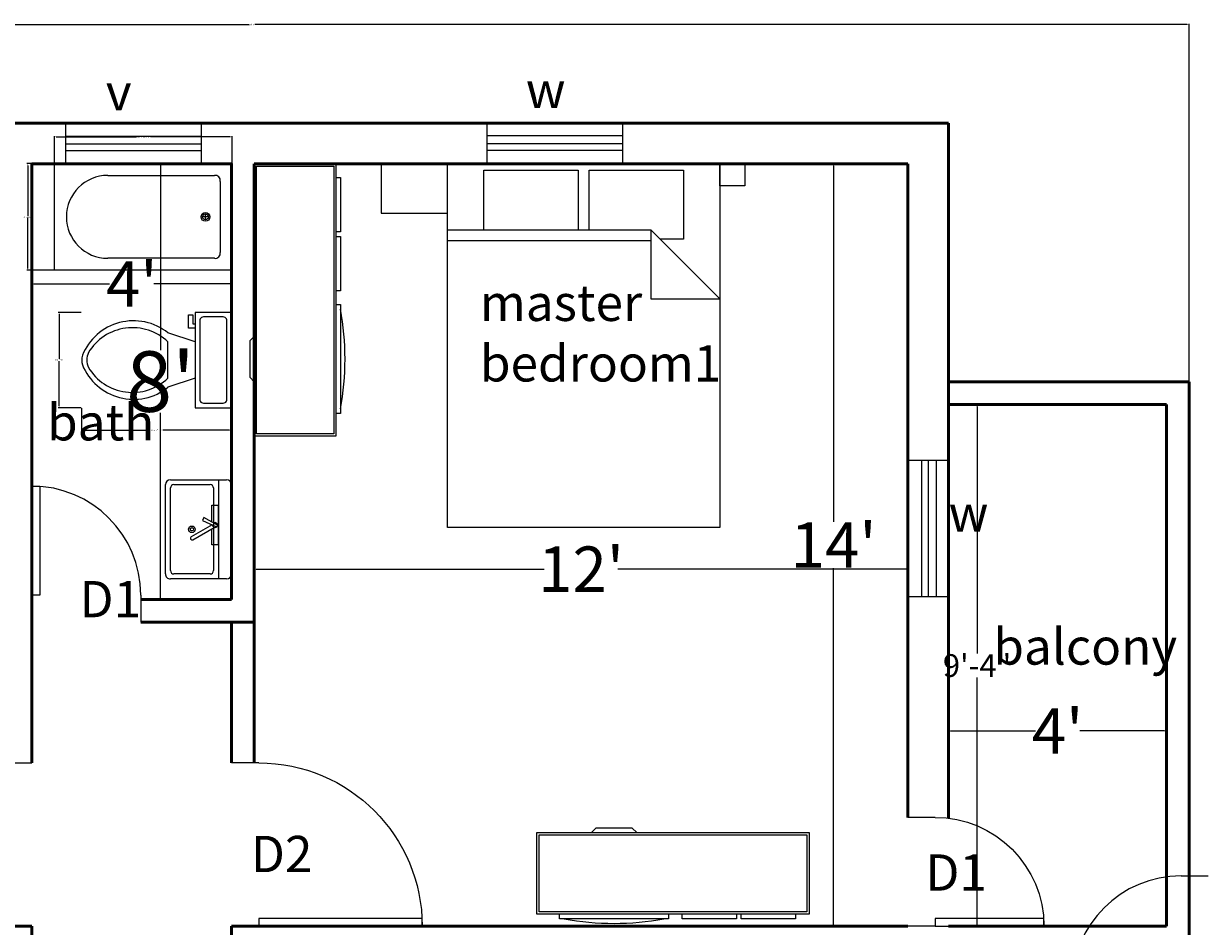
# Model space of a CAD drawing. Units: inches. Extents: x -10 to 557, y -66 to 886.
# Tile 6 of 6: x 210 to 471, y 687 to 886. Entities that reach past the tile are written whole.
import ezdxf

# ---------------------------------------------------------------- set-up
doc = ezdxf.new("R2010")
doc.units = ezdxf.units.IN
doc.header["$MEASUREMENT"] = 0
for name, color, linetype, lineweight in [('A-ANNO-DIMS', 2, 'Continuous', 18), ('A-ANNO-TEXT', 7, 'Continuous', 18), ('A-AREA-IDEN', 7, 'Continuous', 25), ('A-DOOR', 4, 'Continuous', 25), ('A-FLOR-FIXT', 8, 'Continuous', 18), ('A-FURN', 8, 'Continuous', 18), ('A-GLAZ', 4, 'Continuous', 25), ('A-WALL', 7, 'Continuous', 50)]:
    doc.layers.add(name, color=color, linetype=linetype, lineweight=lineweight)
doc.styles.get("Standard").update_dxf_attribs({"font": 'arial.ttf'})
doc.dimstyles.get("Standard").update_dxf_attribs({"dimtxt": 0.3, "dimasz": 0.4, "dimexe": 0.18, "dimexo": 0.0625, "dimgap": 0.09, "dimtad": 0, "dimtih": 1, "dimtoh": 1, "dimdec": 0, "dimrnd": 8, "dimzin": 0, "dimdsep": 46, "dimlunit": 3, "dimtxsty": 'Standard', "dimcen": 0.09, "dimadec": 0, "dimazin": 0, "dimtfac": 1, "dimtdec": 0, "dimtofl": 0, "dimtmove": 0, "dimatfit": 3, "dimfxl": 1, "dimtolj": 1, "dimtzin": 0, "dimarcsym": 0})

# ---------------------------------------------------------------- blocks, each defined once
blk = doc.blocks.new('*U2')
for p, q in [((0, 0), (0, -6)), ((36, 0), (36, -6))]:
    blk.add_line(p, q)
blk.add_lwpolyline([(0, 0), (0, 36), (1.75, 36), (1.75, 0)], close=True)
blk.add_arc((0, 0), 36, 0, 90)
blk = doc.blocks.new('*U3')
for p, q in [((0, 0), (0, -6)), ((24, 0), (24, -6))]:
    blk.add_line(p, q)
blk.add_lwpolyline([(0, 0), (0, 24), (1.75, 24), (1.75, 0)], close=True)
blk.add_arc((0, 0), 24, 0, 90)
blk = doc.blocks.new('*U4')
for p, q in [((0, 0), (0, -6)), ((24, 0), (24, -6))]:
    blk.add_line(p, q)
blk.add_lwpolyline([(0, 0), (0, 24), (1.75, 24), (1.75, 0)], close=True)
blk.add_arc((0, 0), 24, 0, 90)
blk = doc.blocks.new('Bed - Queen')
for p, q in [((0, -80.00003), (0, 0)), ((0, 0), (59.99999, 0)), ((59.99999, 0), (59.99999, -80.00003)), ((7.99999, -1.2), (28.79998, -1.2)), ((7.99999, -14.4), (7.99999, -1.2)), ((28.79998, -1.2), (28.79998, -14.4)), ((31.19999, -1.2), (51.99999, -1.2)), ((31.19999, -14.4), (31.19999, -1.2)), ((51.99999, -1.2), (51.99999, -16.4)), ((0, -14.4), (44.8, -14.4)), ((59.99999, -29.6), (44.8, -14.4)), ((44.8, -14.4), (44.8, -29.6)), ((44.8, -16.8), (0, -16.8)), ((51.99999, -16.4), (46.79936, -16.4)), ((44.8, -29.6), (59.99999, -29.6)), ((59.99999, -80.00003), (0, -80.00003))]:
    blk.add_line(p, q)
blk = doc.blocks.new('Entertainment Center')
for p, q in [((-4, 0), (-5, -1)), ((4, 0), (-4, 0)), ((5, -1), (4, 0)), ((-17, -19), (-17, -1)), ((-17, -1), (43, -1)), ((-16.5, -18.5), (-16.5, -1.5)), ((-16.5, -1.5), (42.5, -1.5)), ((42.5, -1.5), (42.5, -18.5)), ((43, -1), (43, -19)), ((43, -19), (-17, -19)), ((42.5, -18.5), (-16.5, -18.5)), ((-12, -20), (-12, -19)), ((12, -20), (-12, -20)), ((12, -19), (12, -20)), ((15, -20), (15, -19)), ((27, -20), (15, -20)), ((27, -19), (27, -20)), ((28, -20), (28, -19)), ((40, -20), (28, -20)), ((40, -19), (40, -20))]:
    blk.add_line(p, q)
blk.add_arc((0, 40), 61, 259.6111, 280.3889)
blk = doc.blocks.new('Toilet - top')
for p, q in [((9.5, -6), (9.5, -2)), ((-10, -8.5), (-8, -8.5)), ((-10, -9.5), (-10, -8.5)), ((-7, -9.5), (-10, -9.5)), ((-8, -8.5), (-8, -8)), ((-7, -8), (-7, -9.5)), ((-4, -8), (-6, -14)), ((4, -8), (6, -14)), ((4, -14), (-4, -14))]:
    blk.add_line(p, q)
blk.add_lwpolyline([(10.5, -8), (10.5, 0), (-10.5, 0), (-10.5, -8)], close=True)
for points in [[(-9.5, -2), (-9.5, -6)], [(8.5, -1), (-8.5, -1)], [(-8.5, -7), (8.5, -7)]]:
    blk.add_lwpolyline(points)
for centre, radius, start, end in [((-8.62, -1.88), 0.884, 81.8699, 188.1301), ((8.62, -1.88), 0.884, 351.8699, 98.1301), ((-8.62, -6.12), 0.884, 171.8699, 278.1301), ((8.62, -6.12), 0.884, 261.8699, 8.1301), ((3.52, -21.58), 12.17, 141.4691, 247.9714), ((4.2, -21.82), 11.33, 136.3677, 238.9468), ((-3.52, -21.58), 12.17, 292.0284, 38.5307), ((-4.2, -21.82), 11.33, 301.053, 43.6321), ((0, -27.88), 4, 245.7318, 294.2682), ((0, -29), 4, 254.8605, 285.1395)]:
    blk.add_arc(centre, radius, start, end)
blk = doc.blocks.new('Bath Tub - 26 x 60 in.')
for p, q in [((8, -18), (10, -18)), ((9, -17), (9, -19))]:
    blk.add_line(p, q)
blk.add_lwpolyline([(0, -36), (0, 0), (60, 0), (60, -36)], close=True)
for points in [[(6, -4), (42, -4)], [(4, -30), (4, -6)], [(42, -32), (6, -32)]]:
    blk.add_lwpolyline(points)
for radius in [1.5, 1]:
    blk.add_circle((9, -18), radius)
for centre, radius, start, end in [((5.75, -5.75), 1.77, 81.8699, 188.1301), ((42, -18), 14, 270, 90), ((5.75, -30.25), 1.77, 171.8699, 278.1301)]:
    blk.add_arc(centre, radius, start, end)
blk = doc.blocks.new('Sink-single - 30 in top')
blk.add_line((-15, -3.999996), (15, -3.999996))
for points in [[(-13.5, 0), (13.5, 0)], [(-15, -18.499996), (-15, -1.5)], [(15, -1.5), (15, -18.499996)], [(-13.5, -17.499996), (-13.5, -6.499996)], [(-12.5, -5.499996), (12.5, -5.499996)], [(13.5, -6.499996), (13.5, -17.499996)], [(13.5, -19.999996), (-13.5, -19.999996)], [(12.5, -18.499996), (-12.5, -18.499996)]]:
    blk.add_lwpolyline(points)
for radius in [1, 0.5]:
    blk.add_circle((0, -11.999996), radius)
for centre, radius, start, end in [((-13.5, -1.5), 1.5, 90, 180), ((13.5, -1.5), 1.5, 0, 90), ((-12.5, -6.499996), 1, 90, 180), ((12.5, -6.499996), 1, 0, 90), ((-12.5, -17.499996), 1, 180, 270), ((12.5, -17.499996), 1, 270, 0), ((-13.5, -18.499996), 1.5, 180, 270), ((13.5, -18.499996), 1.5, 270, 0)]:
    blk.add_arc(centre, radius, start, end)
blk = doc.blocks.new('Faucet - single handle top')
for p, q in [((0.08, -0.26), (-2.26, -4.34)), ((-1.37, -4.79), (0.55, -0.5)), ((-0.06, -1.9), (3.57, -8.18)), ((4.43, -7.68), (0.72, -1.24)), ((-2.26, -4.34), (-1.37, -4.79))]:
    blk.add_line(p, q)
for points in [[(-0.92, -2), (-6, -2), (-6, 0), (6, 0), (6, -2), (1.16, -2)], [(-0.01, -2), (-0.12, -2)]]:
    blk.add_lwpolyline(points)
for centre, radius, start, end in [((0, -1), 0.75, 269.2246, 216.2304), ((4, -7.93), 0.5, 210, 30)]:
    blk.add_arc(centre, radius, start, end)
blk = doc.blocks.new('*D17')
at = {"layer": 'A-ANNO-DIMS', "color": 0, "lineweight": -2, "transparency": 16777216}
for p, q in [((236.63, 855.28), (240.2, 855.28)), ((240.02, 854.88), (240.02, 814.13)), ((240.02, 759.6), (240.02, 800.34)), ((237.52, 759.2), (240.2, 759.2))]:
    blk.add_line(p, q, dxfattribs=at)
at = {"layer": 'A-ANNO-DIMS', "color": 0, "transparency": 16777216}
for points in [[(239.95, 854.88), (240.08, 854.88), (240.02, 855.28)], [(239.95, 759.6), (240.08, 759.6), (240.02, 759.2)]]:
    blk.add_solid(points, dxfattribs=at)
at = {"layer": 'Defpoints', "color": 0, "transparency": 16777216}
for p in [(236.57, 855.28), (240.02, 855.28), (237.46, 759.2)]:
    blk.add_point(p, dxfattribs=at)
at = {"layer": 'A-ANNO-DIMS', "color": 0, "transparency": 16777216, "insert": (240.02, 807.24), "char_height": 0.3, "attachment_point": 5}
blk.add_mtext("\\A1;{\\H44.44444x;8'}", dxfattribs=at)
blk = doc.blocks.new('*D18')
at = {"layer": 'A-ANNO-DIMS', "color": 0, "lineweight": -2, "transparency": 16777216}
for p, q in [((211.66, 827.66), (211.66, 828.94)), ((212.06, 828.76), (228.77, 828.76)), ((255.26, 828.76), (238.55, 828.76)), ((255.66, 828.55), (255.66, 828.94))]:
    blk.add_line(p, q, dxfattribs=at)
at = {"layer": 'A-ANNO-DIMS', "color": 0, "transparency": 16777216}
for points in [[(212.06, 828.83), (212.06, 828.69), (211.66, 828.76)], [(255.26, 828.83), (255.26, 828.69), (255.66, 828.76)]]:
    blk.add_solid(points, dxfattribs=at)
at = {"layer": 'Defpoints', "color": 0, "transparency": 16777216}
for p in [(211.66, 828.76), (211.66, 827.6), (255.66, 828.49)]:
    blk.add_point(p, dxfattribs=at)
at = {"layer": 'A-ANNO-DIMS', "color": 0, "transparency": 16777216, "insert": (233.66, 828.76), "char_height": 0.3, "attachment_point": 5}
blk.add_mtext("\\A1;{\\H33.33333x;4'}", dxfattribs=at)
blk = doc.blocks.new('*D19')
at = {"layer": 'A-ANNO-DIMS', "color": 0, "lineweight": -2, "transparency": 16777216}
for p, q in [((260.66, 771.19), (260.66, 765.72)), ((404.67, 768.93), (404.67, 765.72)), ((261.06, 765.9), (324.56, 765.9)), ((404.27, 765.9), (340.77, 765.9))]:
    blk.add_line(p, q, dxfattribs=at)
at = {"layer": 'A-ANNO-DIMS', "color": 0, "transparency": 16777216}
for points in [[(261.06, 765.97), (261.06, 765.83), (260.66, 765.9)], [(404.27, 765.97), (404.27, 765.83), (404.67, 765.9)]]:
    blk.add_solid(points, dxfattribs=at)
at = {"layer": 'Defpoints', "color": 0, "transparency": 16777216}
for p in [(260.66, 771.25), (404.67, 768.99), (404.67, 765.9)]:
    blk.add_point(p, dxfattribs=at)
at = {"layer": 'A-ANNO-DIMS', "color": 0, "transparency": 16777216, "insert": (332.67, 765.9), "char_height": 0.3, "attachment_point": 5}
blk.add_mtext("\\A1;{\\H33.33333x;12'}", dxfattribs=at)
blk = doc.blocks.new('*D20')
at = {"layer": 'A-ANNO-DIMS', "color": 0, "lineweight": -2, "transparency": 16777216}
for p, q in [((380.24, 855.2), (388.5, 855.2)), ((388.32, 854.8), (388.32, 776.31)), ((388.32, 687.6), (388.32, 766.09)), ((385.6, 687.2), (388.5, 687.2))]:
    blk.add_line(p, q, dxfattribs=at)
at = {"layer": 'A-ANNO-DIMS', "color": 0, "transparency": 16777216}
for points in [[(388.25, 854.8), (388.38, 854.8), (388.32, 855.2)], [(388.25, 687.6), (388.38, 687.6), (388.32, 687.2)]]:
    blk.add_solid(points, dxfattribs=at)
at = {"layer": 'Defpoints', "color": 0, "transparency": 16777216}
for p in [(380.18, 855.2), (385.54, 687.2), (388.32, 687.2)]:
    blk.add_point(p, dxfattribs=at)
at = {"layer": 'A-ANNO-DIMS', "color": 0, "transparency": 16777216, "insert": (388.32, 771.2), "char_height": 0.3, "attachment_point": 5}
blk.add_mtext("\\A1;{\\H33.33333x;14'}", dxfattribs=at)
blk = doc.blocks.new('*D21')
at = {"layer": 'A-ANNO-DIMS', "color": 0, "lineweight": -2, "transparency": 16777216}
for p, q in [((413.66, 730.3), (413.66, 730.42)), ((414.06, 730.24), (432.77, 730.24)), ((461.26, 730.24), (442.55, 730.24)), ((461.66, 730.3), (461.66, 730.42))]:
    blk.add_line(p, q, dxfattribs=at)
at = {"layer": 'A-ANNO-DIMS', "color": 0, "transparency": 16777216}
for points in [[(414.06, 730.31), (414.06, 730.17), (413.66, 730.24)], [(461.26, 730.31), (461.26, 730.17), (461.66, 730.24)]]:
    blk.add_solid(points, dxfattribs=at)
at = {"layer": 'Defpoints', "color": 0, "transparency": 16777216}
for p in [(413.66, 730.24), (461.66, 730.24), (461.66, 730.24)]:
    blk.add_point(p, dxfattribs=at)
at = {"layer": 'A-ANNO-DIMS', "color": 0, "transparency": 16777216, "insert": (437.66, 730.24), "char_height": 0.3, "attachment_point": 5}
blk.add_mtext("\\A1;{\\H33.33333x;4'}", dxfattribs=at)
blk = doc.blocks.new('*D22')
at = {"layer": 'A-ANNO-DIMS', "color": 0, "lineweight": -2, "transparency": 16777216}
for p, q in [((459.49, 802.16), (419.75, 802.16)), ((419.93, 801.76), (419.93, 747.31)), ((419.93, 687.56), (419.93, 742.02)), ((459.49, 687.16), (419.75, 687.16))]:
    blk.add_line(p, q, dxfattribs=at)
at = {"layer": 'A-ANNO-DIMS', "color": 0, "transparency": 16777216}
for points in [[(419.86, 801.76), (419.99, 801.76), (419.93, 802.16)], [(419.86, 687.56), (419.99, 687.56), (419.93, 687.16)]]:
    blk.add_solid(points, dxfattribs=at)
at = {"layer": 'Defpoints', "color": 0, "transparency": 16777216}
for p in [(459.55, 802.16), (419.93, 687.16), (459.55, 687.16)]:
    blk.add_point(p, dxfattribs=at)
at = {"layer": 'A-ANNO-DIMS', "color": 0, "transparency": 16777216, "insert": (419.93, 744.66), "char_height": 0.3, "attachment_point": 5}
blk.add_mtext('\\A1;{\\H16.66667x;9\'-4"}', dxfattribs=at)
blk = doc.blocks.new('*U31')
for p, q in [((0, 0), (0, -6)), ((24, 0), (24, -6))]:
    blk.add_line(p, q)
blk.add_lwpolyline([(0, 0), (0, 24), (1.75, 24), (1.75, 0)], close=True)
blk.add_arc((0, 0), 24, 0, 90)
blk = doc.blocks.new('WIN-900')
for p, q in [((0, 6.25), (30, 6.25)), ((0, 4.5), (30, 4.5)), ((0, 3.05), (30, 3.05))]:
    blk.add_line(p, q)
blk.add_lwpolyline([(0, 9), (0, 0), (30, 0), (30, 9)], close=True)
blk = doc.blocks.new('*D67')
at = {"layer": 'A-ANNO-DIMS', "color": 0, "lineweight": -2, "ltscale": 2, "transparency": 16777216}
for p, q in [((222.59, 801.41), (222.59, 796.34)), ((255.63, 801.41), (255.63, 796.34)), ((222.99, 796.52), (237.69, 796.52)), ((255.23, 796.52), (240.53, 796.52))]:
    blk.add_line(p, q, dxfattribs=at)
at = {"layer": 'A-ANNO-DIMS', "color": 0, "ltscale": 2, "transparency": 16777216}
for points in [[(222.99, 796.59), (222.99, 796.45), (222.59, 796.52)], [(255.23, 796.59), (255.23, 796.45), (255.63, 796.52)]]:
    blk.add_solid(points, dxfattribs=at)
at = {"layer": 'Defpoints', "color": 0, "ltscale": 2, "transparency": 16777216}
for p in [(222.59, 801.48), (255.63, 801.48), (255.63, 796.52)]:
    blk.add_point(p, dxfattribs=at)
at = {"layer": 'A-ANNO-DIMS', "color": 0, "ltscale": 2, "transparency": 16777216, "insert": (239.11, 796.52), "char_height": 0.3, "attachment_point": 5}
blk.add_mtext('\\A1;WC 2\'-9" TYP.', dxfattribs=at)
blk = doc.blocks.new('*D68')
at = {"layer": 'A-ANNO-DIMS', "color": 0, "lineweight": -2, "ltscale": 2, "transparency": 16777216}
for p, q in [((222.53, 822.48), (217.45, 822.48)), ((217.63, 822.08), (217.63, 812.22)), ((217.63, 801.88), (217.63, 811.73)), ((222.53, 801.48), (217.45, 801.48))]:
    blk.add_line(p, q, dxfattribs=at)
at = {"layer": 'A-ANNO-DIMS', "color": 0, "ltscale": 2, "transparency": 16777216}
for points in [[(217.56, 822.08), (217.7, 822.08), (217.63, 822.48)], [(217.56, 801.88), (217.7, 801.88), (217.63, 801.48)]]:
    blk.add_solid(points, dxfattribs=at)
at = {"layer": 'Defpoints', "color": 0, "ltscale": 2, "transparency": 16777216}
for p in [(222.59, 822.48), (217.63, 801.48), (222.59, 801.48)]:
    blk.add_point(p, dxfattribs=at)
at = {"layer": 'A-ANNO-DIMS', "color": 0, "ltscale": 2, "transparency": 16777216, "insert": (217.63, 811.98), "char_height": 0.3, "attachment_point": 5}
blk.add_mtext('\\A1;1\'-9" TYP.', dxfattribs=at)
blk = doc.blocks.new('*D75')
at = {"layer": 'A-ANNO-DIMS', "color": 0, "lineweight": -2, "ltscale": 2, "transparency": 16777216}
for p, q in [((216.63, 855.34), (216.63, 861.33)), ((217.03, 861.15), (234.62, 861.15)), ((255.37, 861.15), (237.77, 861.15)), ((255.77, 855.34), (255.77, 861.33))]:
    blk.add_line(p, q, dxfattribs=at)
at = {"layer": 'A-ANNO-DIMS', "color": 0, "ltscale": 2, "transparency": 16777216}
for points in [[(217.03, 861.21), (217.03, 861.08), (216.63, 861.15)], [(255.37, 861.21), (255.37, 861.08), (255.77, 861.15)]]:
    blk.add_solid(points, dxfattribs=at)
at = {"layer": 'Defpoints', "color": 0, "ltscale": 2, "transparency": 16777216}
for p in [(216.63, 861.15), (216.63, 855.28), (255.77, 855.28)]:
    blk.add_point(p, dxfattribs=at)
at = {"layer": 'A-ANNO-DIMS', "color": 0, "ltscale": 2, "transparency": 16777216, "insert": (236.2, 861.15), "char_height": 0.3, "attachment_point": 5}
blk.add_mtext('\\A1;BATH TUB 3\'-3"', dxfattribs=at)
blk = doc.blocks.new('*D76')
at = {"layer": 'A-ANNO-DIMS', "color": 0, "lineweight": -2, "ltscale": 2, "transparency": 16777216}
for p, q in [((216.56, 855.28), (210.57, 855.28)), ((210.75, 854.88), (210.75, 843.78)), ((210.75, 832.19), (210.75, 843.29)), ((216.56, 831.79), (210.57, 831.79))]:
    blk.add_line(p, q, dxfattribs=at)
at = {"layer": 'A-ANNO-DIMS', "color": 0, "ltscale": 2, "transparency": 16777216}
for points in [[(210.69, 854.88), (210.82, 854.88), (210.75, 855.28)], [(210.69, 832.19), (210.82, 832.19), (210.75, 831.79)]]:
    blk.add_solid(points, dxfattribs=at)
at = {"layer": 'Defpoints', "color": 0, "ltscale": 2, "transparency": 16777216}
for p in [(216.63, 855.28), (210.75, 831.79), (216.63, 831.79)]:
    blk.add_point(p, dxfattribs=at)
at = {"layer": 'A-ANNO-DIMS', "color": 0, "ltscale": 2, "transparency": 16777216, "insert": (210.75, 843.53), "char_height": 0.3, "attachment_point": 5}
blk.add_mtext('\\A1;1\'-11 1/2"', dxfattribs=at)
blk = doc.blocks.new('*D81')
at = {"layer": 'A-ANNO-DIMS', "color": 0, "lineweight": -2, "ltscale": 2, "transparency": 16777216}
for p, q in [((53.66, 864.26), (53.66, 886.09)), ((54.06, 885.91), (259.56, 885.91)), ((466.26, 885.91), (260.77, 885.91)), ((466.66, 807.26), (466.66, 886.09))]:
    blk.add_line(p, q, dxfattribs=at)
at = {"layer": 'A-ANNO-DIMS', "color": 0, "ltscale": 2, "transparency": 16777216}
for points in [[(54.06, 885.97), (54.06, 885.84), (53.66, 885.91)], [(466.26, 885.97), (466.26, 885.84), (466.66, 885.91)]]:
    blk.add_solid(points, dxfattribs=at)
at = {"layer": 'Defpoints', "color": 0, "ltscale": 2, "transparency": 16777216}
for p in [(466.66, 885.91), (53.66, 864.2), (466.66, 807.2)]:
    blk.add_point(p, dxfattribs=at)
at = {"layer": 'A-ANNO-DIMS', "color": 0, "ltscale": 2, "transparency": 16777216, "insert": (260.16, 885.91), "char_height": 0.3, "attachment_point": 5}
blk.add_mtext('\\A1;34\'-5"', dxfattribs=at)

msp = doc.modelspace()

# ---------------------------------------------------------------- linework, layer by layer
at = {"layer": 'A-FURN'}
for points in [[(303.25, 855.2), (288.58, 855.2), (288.58, 844.33), (303.25, 844.33)], [(363.26, 855.2), (368.79, 855.2), (368.79, 850.39), (363.26, 850.39)]]:
    msp.add_lwpolyline(points, close=True, dxfattribs=at)
at = {"layer": 'A-WALL'}
for p, q in [((53.66, 864.2), (413.66, 864.2)), ((413.66, 864.2), (413.66, 711.01)), ((211.66, 855.2), (255.66, 855.2)), ((211.66, 759.2), (211.66, 855.2)), ((255.66, 855.2), (255.66, 759.2)), ((260.66, 855.2), (260.66, 723.2)), ((260.66, 855.2), (404.66, 855.2)), ((404.66, 855.2), (404.66, 711.2)), ((466.66, 807.2), (413.66, 807.2)), ((466.66, 682.2), (466.66, 807.2)), ((461.66, 802.2), (413.66, 802.2)), ((413.66, 802.2), (413.66, 711.01)), ((461.66, 687.2), (461.66, 802.2)), ((461.66, 802.2), (461.66, 687.2)), ((211.66, 754.2), (211.66, 759.2)), ((235.66, 759.2), (255.66, 759.2)), ((211.66, 723.2), (211.66, 754.2)), ((235.66, 754.2), (260.66, 754.2)), ((255.66, 754.2), (255.66, 723.2)), ((206.66, 687.2), (211.66, 687.2)), ((211.66, 682.2), (211.66, 687.2)), ((260.66, 687.2), (255.66, 687.2)), ((255.66, 687.2), (255.66, 682.2)), ((260.66, 687.2), (404.66, 687.2)), ((413.66, 687.2), (461.66, 687.2))]:
    msp.add_line(p, q, dxfattribs=at)

# ---------------------------------------------------------------- block references
at = {"layer": 'A-DOOR'}
msp.add_blockref('*U3', (211.66, 760.2), dxfattribs=at)
at = {"layer": 'A-DOOR', "rotation": 90}
for name, p in [('*U2', (205.66, 687.2)), ('*U31', (464.89, 674.32))]:
    msp.add_blockref(name, p, dxfattribs=at)
at = {"layer": 'A-DOOR', "xscale": -1, "rotation": 270}
for name, p in [('*U2', (261.66, 687.2)), ('*U4', (410.66, 687.2))]:
    msp.add_blockref(name, p, dxfattribs=at)
at = {"layer": 'A-FLOR-FIXT'}
for name, p, xscale, yscale, zscale, rotation in [('Bath Tub - 26 x 60 in.', (255.77, 831.79), 0.6523347147397875, 0.6523347147397875, 0.6523347147397875, 180), ('Sink-single - 30 in top', (255.66, 774.68), 0.7289455405337706, 0.7289455405337706, 0.7289455405337706, 270), ('Faucet - single handle top', (252.73, 775.62), 0.7289455405337706, 0.7289455405337706, 0.7289455405337706, 270)]:
    msp.add_blockref(name, p, dxfattribs=dict(at, xscale=xscale, yscale=yscale, zscale=zscale, rotation=rotation))
at = {"layer": 'A-FLOR-FIXT', "rotation": 270}
msp.add_blockref('Toilet - top', (255.63, 811.98), dxfattribs=at)
at = {"layer": 'A-FURN', "rotation": 90}
msp.add_blockref('Entertainment Center', (259.66, 812.2), dxfattribs=at)
at = {"layer": 'A-FURN'}
for name, p in [('Bed - Queen', (303.26, 855.05)), ('Entertainment Center', (339.93, 708.85))]:
    msp.add_blockref(name, p, dxfattribs=at)
at = {"layer": 'A-GLAZ'}
for p in [(219.05, 855.1), (311.89, 855.19)]:
    msp.add_blockref('WIN-900', p, dxfattribs=at)
at = {"layer": 'A-GLAZ', "rotation": 270.0000000000005}
msp.add_blockref('WIN-900', (404.67, 789.85), dxfattribs=at)

# ---------------------------------------------------------------- texts
at = {"layer": 'A-ANNO-TEXT', "char_height": 8, "attachment_point": 1}
for s, insert in [('v', (227.94, 875.04)), ('w', (320.49, 875.5)), ('w', (413.67, 782.15)), ('D1', (222.14, 763.29)), ('D2', (259.9, 707.13)), ('D1', (408.54, 703.05))]:
    msp.add_mtext_dynamic_manual_height_columns(s, width=13.506, gutter_width=1, heights=[0], dxfattribs=dict(at, insert=insert))
at = {"layer": 'A-AREA-IDEN', "char_height": 8, "attachment_point": 1}
for s, insert in [(' master bedroom1', (310.38, 828.59)), ('bath', (214.99, 802.27)), ('balcony', (423.51, 752.86))]:
    msp.add_mtext_dynamic_manual_height_columns(s, width=38.1538, gutter_width=1, heights=[0], dxfattribs=dict(at, insert=insert))

# ---------------------------------------------------------------- dimensions: what is measured, and where the dimension line sits
at = {"layer": 'A-ANNO-DIMS', "ltscale": 2}
dim = msp.add_linear_dim(base=(466.66, 885.91), p1=(53.66, 864.2), p2=(466.66, 807.2), dimstyle='Standard', override={"dimdec": 1, "dimlfac": 1, "dimrnd": 0, "dimzin": 1, "dimdsep": 46, "dimlunit": 4, "dimfrac": 2}, dxfattribs=at)
dim.commit()
dim.dimension.update_dxf_attribs({"geometry": '*D81', "text_midpoint": (260.16, 885.91)})
for base, p1, p2, angle, text, picture, middle in [((216.63, 861.15), (255.77, 855.28), (216.63, 855.28), 180, 'BATH TUB <>', '*D75', (236.2, 861.15)), ((217.63, 801.48), (222.59, 822.48), (222.59, 801.48), 270, '<> TYP.', '*D68', (217.63, 811.98))]:
    dim = msp.add_linear_dim(base=base, p1=p1, p2=p2, angle=angle, text=text, dimstyle='Standard', override={"dimdec": 1, "dimrnd": 0, "dimzin": 1, "dimlunit": 4, "dimfrac": 2}, dxfattribs=at)
    dim.commit()
    dim.dimension.update_dxf_attribs({"geometry": picture, "text_midpoint": middle})
dim = msp.add_linear_dim(base=(210.75, 831.79), p1=(216.63, 855.28), p2=(216.63, 831.79), angle=270, dimstyle='Standard', override={"dimdec": 1, "dimrnd": 0, "dimzin": 1, "dimlunit": 4, "dimfrac": 2}, dxfattribs=at)
dim.commit()
dim.dimension.update_dxf_attribs({"geometry": '*D76', "text_midpoint": (210.75, 843.53)})
at = {"layer": 'A-ANNO-DIMS'}
for base, p1, p2, text, picture, middle in [((240.02, 855.28), (237.46, 759.2), (236.57, 855.28), '{\\H44.44444x;<>}', '*D17', (240.02, 807.24)), ((388.32, 687.2), (380.18, 855.2), (385.54, 687.2), '{\\H33.33333x;<>}', '*D20', (388.32, 771.2)), ((419.93, 687.16), (459.55, 802.16), (459.55, 687.16), '{\\H16.66667x;<>}', '*D22', (419.93, 744.66))]:
    dim = msp.add_linear_dim(base=base, p1=p1, p2=p2, angle=90, text=text, dimstyle='Standard', override={"dimclrd": 0, "dimclre": 0, "dimclrt": 0}, dxfattribs=at)
    dim.commit()
    dim.dimension.update_dxf_attribs({"geometry": picture, "text_midpoint": middle})
for base, p1, p2, picture, middle in [((211.66, 828.76), (255.66, 828.49), (211.66, 827.6), '*D18', (233.66, 828.76)), ((404.67, 765.9), (260.66, 771.25), (404.67, 768.99), '*D19', (332.67, 765.9)), ((461.66, 730.24), (413.66, 730.24), (461.66, 730.24), '*D21', (437.66, 730.24))]:
    dim = msp.add_linear_dim(base=base, p1=p1, p2=p2, text='{\\H33.33333x;<>}', dimstyle='Standard', override={"dimclrd": 0, "dimclre": 0, "dimclrt": 0}, dxfattribs=at)
    dim.commit()
    dim.dimension.update_dxf_attribs({"geometry": picture, "text_midpoint": middle})
at = {"layer": 'A-ANNO-DIMS', "ltscale": 2}
dim = msp.add_linear_dim(base=(255.63, 796.52), p1=(222.59, 801.48), p2=(255.63, 801.48), text='WC <> TYP.', dimstyle='Standard', override={"dimdec": 1, "dimrnd": 0, "dimzin": 1, "dimlunit": 4, "dimfrac": 2}, dxfattribs=at)
dim.commit()
dim.dimension.update_dxf_attribs({"geometry": '*D67', "text_midpoint": (239.11, 796.52)})

doc.saveas('drawing.dxf')
